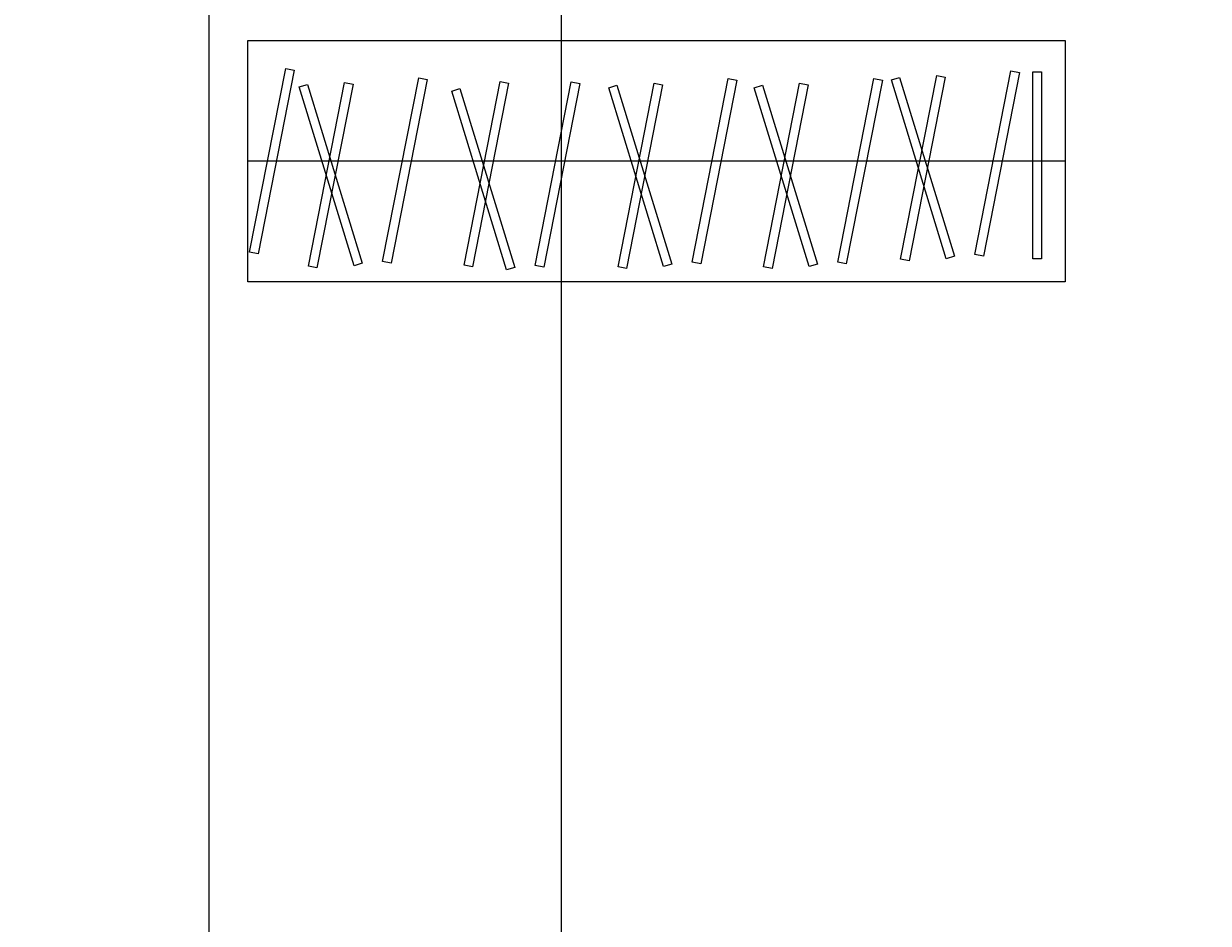
# Model space of a CAD drawing. Units: inches. Extents: x -61 to 1599, y -1316 to 257.
# Tile 91 of 204: x 240 to 321, y -280 to -219. Entities that reach past the tile are written whole.
import ezdxf

# ---------------------------------------------------------------- set-up
doc = ezdxf.new("R2010")
doc.units = ezdxf.units.IN
doc.header["$MEASUREMENT"] = 0
doc.layers.add('A-ANNO-DIMS', color=2, linetype='Continuous', lineweight=18)
doc.layers.add('A-FLOR-CASE', color=8, linetype='Continuous', lineweight=18)
doc.styles.get("Standard").update_dxf_attribs({"font": 'arial.ttf'})
doc.dimstyles.get("Standard").update_dxf_attribs({"dimtxt": 0.18, "dimasz": 0.18, "dimexe": 0.18, "dimexo": 0.0625, "dimgap": 0.09, "dimtad": 0, "dimtih": 1, "dimtoh": 1, "dimdec": 0, "dimzin": 0, "dimdsep": 46, "dimlunit": 3, "dimtxsty": 'Standard', "dimcen": 0.09, "dimadec": 0, "dimazin": 0, "dimtfac": 1, "dimtdec": 0, "dimtofl": 0, "dimtmove": 0, "dimatfit": 3, "dimfxl": 1, "dimtolj": 1, "dimtzin": 0, "dimarcsym": 0})

# ---------------------------------------------------------------- blocks, each defined once
blk = doc.blocks.new('WARDROBE-HANGING-2')
blk.add_line((55.703, 8.23), (0, 8.23))
for points in [[(55.703, 16.46), (55.703, 0), (0, 0), (0, 16.46)], [(0.121, 2.033), (2.581, 14.541), (3.16, 14.427), (0.7, 1.92)], [(9.187, 1.403), (11.648, 13.911), (12.226, 13.797), (9.766, 1.289)], [(30.284, 1.352), (32.745, 13.859), (33.323, 13.745), (30.863, 1.238)], [(40.204, 1.348), (42.664, 13.855), (43.243, 13.742), (40.782, 1.234)], [(47.6, 1.579), (43.858, 13.764), (44.421, 13.937), (48.164, 1.752)], [(44.491, 1.561), (46.952, 14.069), (47.53, 13.955), (45.07, 1.448)], [(49.548, 1.88), (52.008, 14.387), (52.587, 14.273), (50.127, 1.766)], [(54.096, 14.328), (54.096, 1.581), (53.506, 1.581), (53.506, 14.328)], [(7.24, 1.102), (3.497, 13.288), (4.061, 13.461), (7.804, 1.276)], [(4.131, 1.085), (6.591, 13.592), (7.17, 13.478), (4.709, 0.971)], [(17.639, 0.817), (13.896, 13.002), (14.46, 13.175), (18.203, 0.99)], [(14.733, 1.142), (17.193, 13.649), (17.772, 13.535), (15.312, 1.028)], [(19.586, 1.118), (22.047, 13.625), (22.625, 13.511), (20.165, 1.004)], [(28.337, 1.051), (24.594, 13.236), (25.158, 13.409), (28.901, 1.224)], [(25.228, 1.034), (27.688, 13.541), (28.267, 13.427), (25.806, 0.92)], [(38.256, 1.047), (34.513, 13.232), (35.077, 13.406), (38.82, 1.221)], [(35.147, 1.03), (37.607, 13.537), (38.186, 13.423), (35.726, 0.916)]]:
    blk.add_lwpolyline(points, close=True)
blk = doc.blocks.new('*D687')
at = {"layer": 'A-ANNO-DIMS', "color": 0, "lineweight": -2, "transparency": 16777216}
for p, q in [((289.418, 181.677), (-61.077, 181.677)), ((-60.897, 181.497), (-60.897, -528.952)), ((-60.897, -1239.765), (-60.897, -529.316)), ((319.64, -1239.945), (-61.077, -1239.945))]:
    blk.add_line(p, q, dxfattribs=at)
at = {"layer": 'A-ANNO-DIMS', "color": 0, "transparency": 16777216}
for points in [[(-60.927, 181.497), (-60.867, 181.497), (-60.897, 181.677)], [(-60.927, -1239.765), (-60.867, -1239.765), (-60.897, -1239.945)]]:
    blk.add_solid(points, dxfattribs=at)
at = {"layer": 'DEFPOINTS', "color": 0, "transparency": 16777216}
for p in [(289.481, 181.677), (-60.897, -1239.945), (319.703, -1239.945)]:
    blk.add_point(p, dxfattribs=at)
at = {"layer": 'A-ANNO-DIMS', "color": 0, "transparency": 16777216, "insert": (-60.897, -529.134), "char_height": 0.18, "attachment_point": 5}
blk.add_mtext('\\A1;1421.6', dxfattribs=at)
blk = doc.blocks.new('*D699')
at = {"layer": 'A-ANNO-DIMS', "color": 0, "lineweight": -2, "transparency": 16777216}
for p, q in [((835.64, -167.169), (-61.077, -167.169)), ((-60.897, -167.349), (-60.897, -306.726)), ((-60.897, -446.466), (-60.897, -307.09)), ((841.64, -446.646), (-61.077, -446.646))]:
    blk.add_line(p, q, dxfattribs=at)
at = {"layer": 'A-ANNO-DIMS', "color": 0, "transparency": 16777216}
for points in [[(-60.927, -167.349), (-60.867, -167.349), (-60.897, -167.169)], [(-60.927, -446.466), (-60.867, -446.466), (-60.897, -446.646)]]:
    blk.add_solid(points, dxfattribs=at)
at = {"layer": 'DEFPOINTS', "color": 0, "transparency": 16777216}
for p in [(835.703, -167.169), (-60.897, -446.646), (841.703, -446.646)]:
    blk.add_point(p, dxfattribs=at)
at = {"layer": 'A-ANNO-DIMS', "color": 0, "transparency": 16777216, "insert": (-60.897, -306.908), "char_height": 0.18, "attachment_point": 5}
blk.add_mtext('\\A1;279.5', dxfattribs=at)
blk = doc.blocks.new('*D701')
at = {"layer": 'A-ANNO-DIMS', "color": 0, "lineweight": -2, "transparency": 16777216}
for p, q in [((215.752, -616.882), (215.752, 257.457)), ((215.932, 257.277), (233.924, 257.277)), ((252.702, 257.277), (234.711, 257.277)), ((252.882, -616.882), (252.882, 257.457))]:
    blk.add_line(p, q, dxfattribs=at)
at = {"layer": 'A-ANNO-DIMS', "color": 0, "transparency": 16777216}
for points in [[(215.932, 257.307), (215.932, 257.247), (215.752, 257.277)], [(252.702, 257.307), (252.702, 257.247), (252.882, 257.277)]]:
    blk.add_solid(points, dxfattribs=at)
at = {"layer": 'DEFPOINTS', "color": 0, "transparency": 16777216}
for p in [(252.882, 257.277), (215.752, -616.945), (252.882, -616.945)]:
    blk.add_point(p, dxfattribs=at)
at = {"layer": 'A-ANNO-DIMS', "color": 0, "transparency": 16777216, "insert": (234.317, 257.277), "char_height": 0.18, "attachment_point": 5}
blk.add_mtext('\\A1;37.13', dxfattribs=at)
blk = doc.blocks.new('*D702')
at = {"layer": 'A-ANNO-DIMS', "color": 0, "lineweight": -2, "transparency": 16777216}
for p, q in [((276.882, -616.882), (276.882, 257.457)), ((277.062, 257.277), (312.209, 257.277)), ((348.14, 257.277), (312.994, 257.277)), ((348.32, -616.882), (348.32, 257.457))]:
    blk.add_line(p, q, dxfattribs=at)
at = {"layer": 'A-ANNO-DIMS', "color": 0, "transparency": 16777216}
for points in [[(277.062, 257.307), (277.062, 257.247), (276.882, 257.277)], [(348.14, 257.307), (348.14, 257.247), (348.32, 257.277)]]:
    blk.add_solid(points, dxfattribs=at)
at = {"layer": 'DEFPOINTS', "color": 0, "transparency": 16777216}
for p in [(348.32, 257.277), (276.882, -616.945), (348.32, -616.945)]:
    blk.add_point(p, dxfattribs=at)
at = {"layer": 'A-ANNO-DIMS', "color": 0, "transparency": 16777216, "insert": (312.601, 257.277), "char_height": 0.18, "attachment_point": 5}
blk.add_mtext('\\A1;71.44', dxfattribs=at)

msp = doc.modelspace()

# ---------------------------------------------------------------- block references
at = {"layer": 'A-FLOR-CASE'}
msp.add_blockref('WARDROBE-HANGING-2', (255.5089, -236.2253), dxfattribs=at)

# ---------------------------------------------------------------- dimensions: what is measured, and where the dimension line sits
at = {"layer": 'A-ANNO-DIMS'}
for base, p1, p2, picture, middle in [((252.8825, 257.2771), (215.7521, -616.9446), (252.8825, -616.9446), '*D701', (234.3173, 257.2771)), ((348.3201, 257.2771), (276.8825, -616.9446), (348.3201, -616.9446), '*D702', (312.6013, 257.2771))]:
    dim = msp.add_linear_dim(base=base, p1=p1, p2=p2, dimstyle='Standard', override={"dimdec": 2, "dimlfac": 1, "dimrnd": 0, "dimzin": 0, "dimdsep": 46, "dimlunit": 2}, dxfattribs=at)
    dim.commit()
    dim.dimension.update_dxf_attribs({"geometry": picture, "text_midpoint": middle})
for base, p1, p2, picture, middle in [((-60.8972, -1239.9446), (289.4807, 181.6771), (319.7028, -1239.9446), '*D687', (-60.8972, -529.1337)), ((-60.8972, -446.6462), (835.7028, -167.169), (841.7028, -446.6462), '*D699', (-60.8972, -306.9076))]:
    dim = msp.add_linear_dim(base=base, p1=p1, p2=p2, angle=90, dimstyle='Standard', override={"dimdec": 1, "dimlfac": 1, "dimrnd": 0, "dimzin": 0, "dimdsep": 46, "dimlunit": 2}, dxfattribs=at)
    dim.commit()
    dim.dimension.update_dxf_attribs({"geometry": picture, "text_midpoint": middle})

doc.saveas('drawing.dxf')
